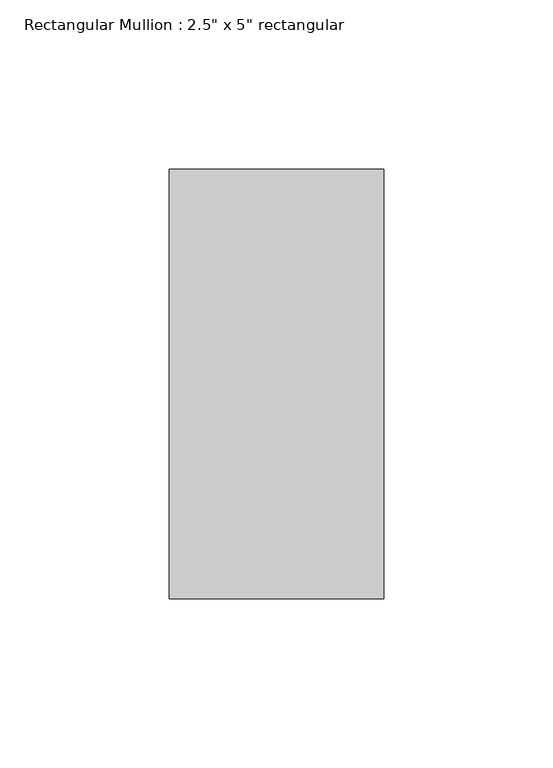
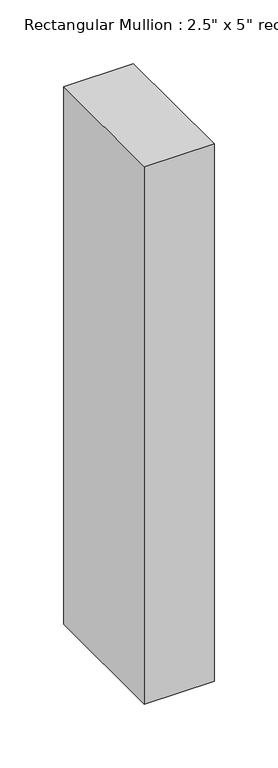
"""IFC4 building model written with IfcOpenShell, lengths in millimetres: member geometry."""

from ifc_helpers import new_model, si_unit, frame, origin, place, context, project, spatial, polyline, outline, extrude, source, transform, mapped, element, save


def member_ce4f90f2(model_context):
    return source(origin(), model_context, "Body", "SweptSolid", [
        extrude(outline(polyline([(0.0, 63.5), (0.0, -63.5), (-63.5, -63.5), (-63.5, 63.5), (0.0, 63.5)])), frame((0.0, 0.0, -516.4666667), z_axis=(0.0, 0.0, 1.0), x_axis=(1.0, 0.0, 0.0)), (0.0, 0.0, 1.0), 516.4666667),
    ])


if __name__ == "__main__":
    model = new_model("IFC4")
    model_context = context("Model", 3, world=origin())
    ifc_project = project(units=[si_unit("LENGTHUNIT", "METRE", prefix="MILLI")], contexts=[model_context])
    site = spatial("IfcSite", under=ifc_project)
    building = spatial("IfcBuilding", under=site)
    placement = place(None, origin())
    member_shape = member_ce4f90f2(model_context)
    element("IfcMember", 1, ObjectType="Rectangular Mullion : 2.5\" x 5\" rectangular", at=placement, inside=building, context=model_context, shape_type="MappedRepresentation", body=[
        mapped(member_shape, transform((0.0, 0.0, 0.0), x_axis=(1.0, 0.0, 0.0), y_axis=(0.0, 1.0, 0.0), z_axis=(0.0, 0.0, 1.0))),
    ])
    save(model, "model.ifc")

# Revit data of these elements
# Type "Rectangular Mullion : 2.5\" x 5\" rectangular"
#   built-in parameter 1007304 = 0.416667 (stored number, unit not read)
#   built-in parameter 1007301 = 0.104167 (stored number, unit not read)
#   built-in parameter 1007300 = 0.104167 (stored number, unit not read)
# Element 1 (IfcMember, "Rectangular Mullion : 2.5\" x 5\" rectangular")
#   Materials on its faces: "Aluminum"
# Materials
#   "Aluminum": class "Metal", colour RGB 247 247 247, transparency 0, Description = "Aluminum 6061", Cost = 0
